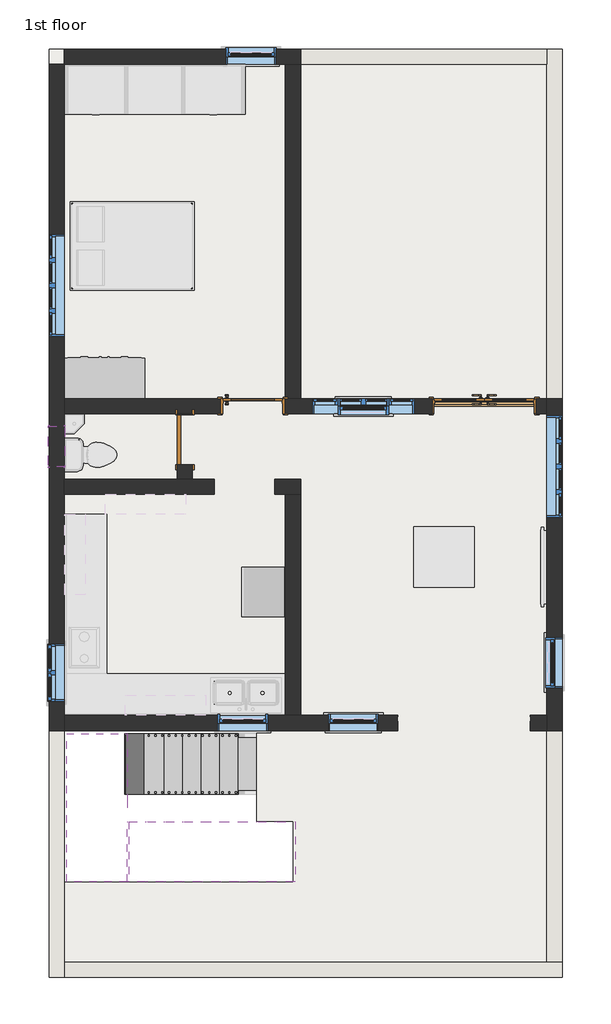
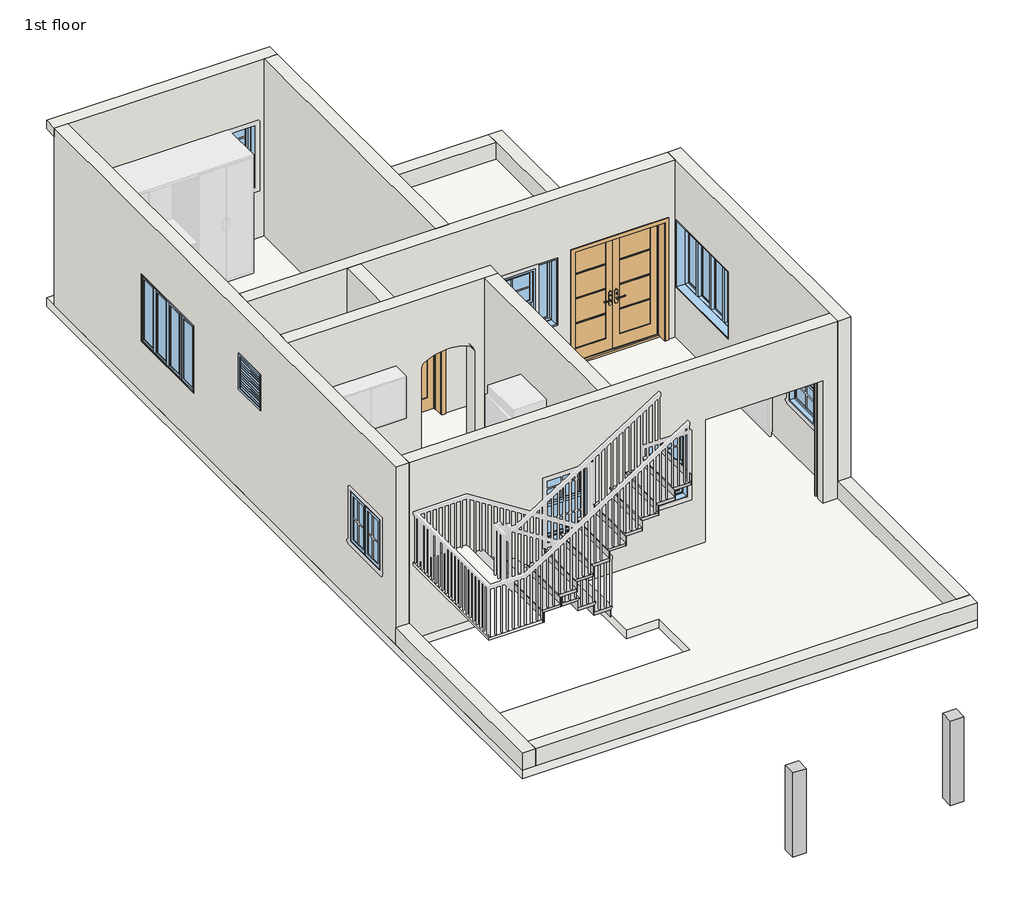
# One storey, part 1 of 3: 14 walls, 10 windows, 3 doors, 2 columns, 2 slabs, 2 stair flights.
"""IFC4 building model written with IfcOpenShell, lengths in millimetres."""

from ifc_helpers import new_model, si_unit, point, frame, origin, place, context, project, spatial, polyline, ellipse_curve, trimmed, outline, extrude, faceted_brep, transform, mapped, element, save
from ifc_brep_helpers import plane_surface, extruded_surface, advanced_brep
from components import concrete_square_column_fdf53bfc, door_7bc300fe, door_3b97b8e7, door_bb98abfd, non_monolithic_landing_a0269062, stair_flight_80511569, stair_flight_9ab9eb73, window_339605e1, window_cf6260c5, window_d400040f, window_913990a0, window_f2d8fef0

model = new_model("IFC4")

# Units and contexts
model_context = context("Model", 3, world=origin())
ifc_project = project(units=[si_unit("LENGTHUNIT", "METRE", prefix="MILLI")], contexts=[model_context])

# Site, building, storey
site = spatial("IfcSite", under=ifc_project)
building = spatial("IfcBuilding", under=site)
storey = spatial("IfcBuildingStorey", under=building, Name="1st floor", Elevation=3810.0)

# Columns
placement = place(None, origin())
concrete_square_column_shape = concrete_square_column_fdf53bfc(model_context)
element("IfcColumn", 1, ObjectType="Concrete-Square-Column", at=placement, inside=storey, context=model_context, shape_type="MappedRepresentation", body=[
    mapped(concrete_square_column_shape, transform((35811.8316163, 5713.6980552, 0.0), x_axis=(1.0, 0.0, 0.0), y_axis=(0.0, 1.0, 0.0), z_axis=(0.0, 0.0, 1.0))),
])
element("IfcColumn", 2, ObjectType="Concrete-Square-Column", at=placement, inside=storey, context=model_context, shape_type="MappedRepresentation", body=[
    mapped(concrete_square_column_shape, transform((33125.7468179, 5719.9369036, 0.0), x_axis=(1.0, 0.0, 0.0), y_axis=(0.0, 1.0, 0.0), z_axis=(0.0, 0.0, 1.0))),
])

# Doors
door_shape = door_7bc300fe(model_context)
element("IfcDoor", 3, ObjectType="Door-Exterior-Double-Full Glass-Wood_Clad : 60\" x 84\"", at=placement, inside=storey, context=model_context, shape_type="MappedRepresentation", body=[
    mapped(door_shape, transform((34973.6316163, 14251.2730552, 3810.0), x_axis=(-1.0, 0.0, 0.0), y_axis=(0.0, -1.0, 0.0), z_axis=(0.0, 0.0, 1.0))),
])
door_2_shape = door_3b97b8e7(model_context)
element("IfcDoor", 4, ObjectType="Door-Interior-Single-1_Panel-Wood : 36\" x 84\"", at=placement, inside=storey, context=model_context, shape_type="MappedRepresentation", body=[
    mapped(door_2_shape, transform((31468.4316163, 14251.2730552, 3810.0), x_axis=(1.0, 0.0, 0.0), y_axis=(0.0, 1.0, 0.0), z_axis=(0.0, 0.0, 1.0))),
])
door_3_shape = door_bb98abfd(model_context)
element("IfcDoor", 5, ObjectType="Single-Flush : 30\" x 84\"", at=placement, inside=storey, context=model_context, shape_type="MappedRepresentation", body=[
    mapped(door_3_shape, transform((30439.7316163, 13740.0980552, 3810.0), x_axis=(0.0, 1.0, 0.0), y_axis=(-1.0, 0.0, 0.0), z_axis=(0.0, 0.0, 1.0))),
])

# Slabs
element("IfcSlab", 6, ObjectType="Generic - 12\" 2", at=placement, inside=storey, context=model_context, shape_type="SweptSolid", body=[
    extrude(outline(polyline([(36154.7316163, 19658.2980552), (36154.7316163, 5593.0480552), (28382.3316163, 5593.0480552), (28382.3316163, 19658.2980552), (36154.7316163, 19658.2980552)]), holes=[polyline([(31519.2316163, 7955.2480552), (31519.2316163, 9333.1980552), (28610.9316163, 9333.1980552), (28610.9316163, 7040.8480552), (32078.0316163, 7040.8480552), (32078.0316163, 7955.2480552), (31519.2316163, 7955.2480552)])]), frame((0.0, 0.0, 3657.6), z_axis=(0.0, 0.0, 1.0), x_axis=(1.0, 0.0, 0.0)), (0.0, 0.0, 1.0), 152.4),
])
non_monolithic_landing_shape = non_monolithic_landing_a0269062(model_context)
element("IfcSlab", 7, ObjectType="Non-Monolithic Landing", at=placement, inside=storey, context=model_context, shape_type="MappedRepresentation", body=[
    mapped(non_monolithic_landing_shape, transform((0.0, 0.0, 0.0), x_axis=(1.0, 0.0, 0.0), y_axis=(0.0, 1.0, 0.0), z_axis=(0.0, 0.0, 1.0))),
])

# Stair flights
stair_flight_shape = stair_flight_80511569(model_context)
element("IfcStairFlight", 8, ObjectType="2\" Tread 1\" Nosing 1/4\" Riser", at=placement, inside=storey, context=model_context, shape_type="MappedRepresentation", body=[
    mapped(stair_flight_shape, transform((0.0, 0.0, 0.0), x_axis=(1.0, 0.0, 0.0), y_axis=(0.0, 1.0, 0.0), z_axis=(0.0, 0.0, 1.0))),
])
stair_flight_2_shape = stair_flight_9ab9eb73(model_context)
element("IfcStairFlight", 9, ObjectType="2\" Tread 1\" Nosing 1/4\" Riser", at=placement, inside=storey, context=model_context, shape_type="MappedRepresentation", body=[
    mapped(stair_flight_2_shape, transform((0.0, 0.0, 0.0), x_axis=(1.0, 0.0, 0.0), y_axis=(0.0, 1.0, 0.0), z_axis=(0.0, 0.0, 1.0))),
])

# Walls
element("IfcWall", 10, ObjectType="Generic - 9\"", at=placement, inside=storey, context=model_context, shape_type="Brep", body=[
    faceted_brep([(28610.9316163, 19429.6980552, 3810.0), (31963.7316163, 19429.6980552, 3810.0), (32192.3316163, 19429.6980552, 3810.0), (32192.3316163, 19429.6980552, 4114.8), (32192.3316163, 19429.6980552, 7010.4), (31963.7316163, 19429.6980552, 7010.4), (28610.9316163, 19429.6980552, 7010.4), (28382.3316163, 19429.6980552, 7010.4), (28382.3316163, 19429.6980552, 6858.0), (28610.9316163, 19429.6980552, 6858.0), (31062.0316163, 19429.6980552, 5892.8), (31824.0316163, 19429.6980552, 5892.8), (31824.0316163, 19429.6980552, 4724.4), (31062.0316163, 19429.6980552, 4724.4), (28610.9316163, 19658.2980552, 3810.0), (28610.9316163, 19658.2980552, 6858.0), (28382.3316163, 19658.2980552, 6858.0), (28382.3316163, 19658.2980552, 7010.4), (32192.3316163, 19658.2980552, 7010.4), (32192.3316163, 19658.2980552, 4114.8), (32192.3316163, 19658.2980552, 3810.0), (31062.0316163, 19658.2980552, 5892.8), (31062.0316163, 19658.2980552, 4724.4), (31824.0316163, 19658.2980552, 4724.4), (31824.0316163, 19658.2980552, 5892.8)], [[[0, 1, 2, 3, 4, 5, 6, 7, 8, 9], [10, 11, 12, 13]], [[14, 15, 16, 17, 18, 19, 20], [21, 22, 23, 24]], [[2, 1, 0, 14, 20]], [[7, 6, 5, 4, 18, 17]], [[22, 21, 10, 13]], [[23, 22, 13, 12]], [[24, 23, 12, 11]], [[21, 24, 11, 10]], [[2, 20, 19, 18, 4, 3]], [[8, 16, 15, 9]], [[0, 9, 15, 14]], [[8, 7, 17, 16]]]),
])
element("IfcWall", 11, ObjectType="Generic - 9\"", at=placement, inside=storey, context=model_context, shape_type="Brep", body=[
    faceted_brep([(35926.1316163, 14133.7980552, 7010.4), (30554.0316163, 14133.7980552, 7010.4), (30325.4316163, 14133.7980552, 7010.4), (28610.9316163, 14133.7980552, 7010.4), (28610.9316163, 14133.7980552, 3810.0), (30325.4316163, 14133.7980552, 3810.0), (30554.0316163, 14133.7980552, 3810.0), (30985.8316163, 14133.7980552, 3810.0), (30985.8316163, 14133.7980552, 5969.0), (31951.0316163, 14133.7980552, 5969.0), (31951.0316163, 14133.7980552, 3810.0), (34186.2316163, 14133.7980552, 3810.0), (34186.2316163, 14133.7980552, 5969.0), (35761.0316163, 14133.7980552, 5969.0), (35761.0316163, 14133.7980552, 3810.0), (35926.1316163, 14133.7980552, 3810.0), (33919.5316163, 14133.7980552, 4724.4), (32370.1316163, 14133.7980552, 4724.4), (32370.1316163, 14133.7980552, 5943.6), (33919.5316163, 14133.7980552, 5943.6), (28610.9316163, 14362.3980552, 7010.4), (31963.7316163, 14362.3980552, 7010.4), (32192.3316163, 14362.3980552, 7010.4), (35926.1316163, 14362.3980552, 7010.4), (35926.1316163, 14362.3980552, 6858.0), (35926.1316163, 14362.3980552, 3810.0), (35761.0316163, 14362.3980552, 3810.0), (35761.0316163, 14362.3980552, 5969.0), (34186.2316163, 14362.3980552, 5969.0), (34186.2316163, 14362.3980552, 3810.0), (32192.3316163, 14362.3980552, 3810.0), (31963.7316163, 14362.3980552, 3810.0), (31951.0316163, 14362.3980552, 3810.0), (31951.0316163, 14362.3980552, 5969.0), (30985.8316163, 14362.3980552, 5969.0), (30985.8316163, 14362.3980552, 3810.0), (28610.9316163, 14362.3980552, 3810.0), (32370.1316163, 14362.3980552, 4724.4), (33919.5316163, 14362.3980552, 4724.4), (33919.5316163, 14362.3980552, 5943.6), (32370.1316163, 14362.3980552, 5943.6)], [[[0, 1, 2, 3, 4, 5, 6, 7, 8, 9, 10, 11, 12, 13, 14, 15], [16, 17, 18, 19]], [[20, 21, 22, 23, 24, 25, 26, 27, 28, 29, 30, 31, 32, 33, 34, 35, 36], [37, 38, 39, 40]], [[4, 36, 35, 7, 6, 5]], [[15, 14, 26, 25]], [[29, 11, 10, 32, 31, 30]], [[3, 2, 1, 0, 23, 22, 21, 20]], [[37, 17, 16, 38]], [[28, 12, 11, 29]], [[12, 28, 27, 13]], [[13, 27, 26, 14]], [[9, 33, 32, 10]], [[33, 9, 8, 34]], [[34, 8, 7, 35]], [[19, 39, 38, 16]], [[17, 37, 40, 18]], [[39, 19, 18, 40]], [[15, 25, 24, 23, 0]], [[3, 20, 36, 4]]]),
])
element("IfcWall", 12, ObjectType="Generic - 9\"", at=placement, inside=storey, context=model_context, shape_type="AdvancedBrep", body=[
    advanced_brep(
    [(28610.9316163, 12914.5980552, 3810.0), (30884.2316163, 12914.5980552, 3810.0), (30884.2316163, 12914.5980552, 5740.4), (31798.6316163, 12914.5980552, 5740.4), (31798.6316163, 12914.5980552, 3810.0), (31963.7316163, 12914.5980552, 3810.0), (32192.3316163, 12914.5980552, 3810.0), (32192.3316163, 12914.5980552, 6858.0), (32192.3316163, 12914.5980552, 7010.4), (31963.7316163, 12914.5980552, 7010.4), (28610.9316163, 12914.5980552, 7010.4), (30884.2316163, 13143.1980552, 5740.4), (30884.2316163, 13143.1980552, 3810.0), (30554.0316163, 13143.1980552, 3810.0), (30325.4316163, 13143.1980552, 3810.0), (28610.9316163, 13143.1980552, 3810.0), (28610.9316163, 13143.1980552, 7010.4), (30325.4316163, 13143.1980552, 7010.4), (30554.0316163, 13143.1980552, 7010.4), (32192.3316163, 13143.1980552, 7010.4), (32192.3316163, 13143.1980552, 3810.0), (31963.7316163, 13143.1980552, 3810.0), (31798.6316163, 13143.1980552, 3810.0), (31798.6316163, 13143.1980552, 5740.4)],
    [
        (0, 1),
        (1, 2),
        (2, 3, ellipse_curve(frame((31341.4316163, 12914.5980552, 5740.4), z_axis=(0.0, 1.0, 0.0), x_axis=(-1.0, 0.0, 0.0)), 457.2, 203.2)),
        (3, 4),
        (4, 5),
        (5, 6),
        (6, 7),
        (7, 8),
        (8, 9),
        (9, 10),
        (10, 0),
        (11, 12),
        (12, 13),
        (13, 14),
        (14, 15),
        (15, 16),
        (16, 17),
        (17, 18),
        (18, 19),
        (19, 20),
        (20, 21),
        (21, 22),
        (22, 23),
        (23, 11, ellipse_curve(frame((31341.4316163, 13143.1980552, 5740.4), z_axis=(0.0, -1.0, 0.0), x_axis=(-1.0, 0.0, 0.0)), 457.2, 203.2)),
        (12, 1),
        (0, 15),
        (20, 6),
        (4, 22),
        (8, 19),
        (16, 10),
        (2, 11),
        (23, 3),
    ],
    [
        plane_surface(frame((28648.9011308, 12914.5980552, 3810.0), z_axis=(0.0, -1.0, 0.0), x_axis=(1.0, 0.0, 0.0))),
        plane_surface(frame((28648.9011308, 13143.1980552, 3810.0), z_axis=(0.0, 1.0, 0.0), x_axis=(-1.0, 0.0, 0.0))),
        plane_surface(frame((28496.6316163, 12914.5980552, 3810.0), z_axis=(0.0, 0.0, -1.0), x_axis=(0.0, 1.0, 0.0))),
        plane_surface(frame((32078.0316163, 12914.5980552, 7010.4), z_axis=(0.0, 0.0, 1.0), x_axis=(0.0, 1.0, 0.0))),
        plane_surface(frame((28610.9316163, 5713.6980552, 3810.0), z_axis=(-1.0, 0.0, 0.0), x_axis=(0.0, 1.0, 0.0))),
        extruded_surface(trimmed(ellipse_curve(frame((31341.4316163, 13371.7980552, 5740.4), z_axis=(0.0, 1.0, 0.0), x_axis=(-1.0, 0.0, 0.0)), 457.2, 203.2), [point((30884.2316163, 13371.7980552, 5740.4))], [point((31798.6316163, 13371.7980552, 5740.4))], True, "CARTESIAN"), (0.0, -228.60000000000036, 0.0), 228.60000000000036),
        plane_surface(frame((31798.6316163, 12914.5980552, 5740.4), z_axis=(-1.0, 0.0, 0.0), x_axis=(0.0, 1.0, 0.0))),
        plane_surface(frame((30884.2316163, 12914.5980552, 3810.0), z_axis=(1.0, 0.0, 0.0), x_axis=(0.0, 1.0, 0.0))),
        plane_surface(frame((32192.3316163, 9561.7980552, 3810.0), z_axis=(1.0, 0.0, 0.0), x_axis=(0.0, 1.0, 0.0))),
    ],
    [
        (0, [[1, 2, 3, 4, 5, 6, 7, 8, 9, 10, 11]]),
        (1, [[12, 13, 14, 15, 16, 17, 18, 19, 20, 21, 22, 23, 24]]),
        (2, [[-15, -14, -13, 25, -1, 26]]),
        (2, [[-22, -21, 27, -6, -5, 28]]),
        (3, [[-10, -9, 29, -19, -18, -17, 30]]),
        (4, [[-11, -30, -16, -26]]),
        (5, [[-3, 31, -24, 32]]),
        (6, [[-4, -32, -23, -28]]),
        (7, [[-2, -25, -12, -31]]),
        (8, [[-27, -20, -29, -8, -7]]),
    ],
),
])
element("IfcWall", 13, ObjectType="Generic - 9\"", at=placement, inside=storey, context=model_context, shape_type="Brep", body=[
    faceted_brep([(35926.1316163, 9333.1980552, 7010.4), (28610.9316163, 9333.1980552, 7010.4), (28610.9316163, 9333.1980552, 3810.0), (33668.8316163, 9333.1980552, 3810.0), (33668.8316163, 9333.1980552, 6019.0), (35668.8316163, 9333.1980552, 6019.0), (35668.8316163, 9333.1980552, 3810.0), (35926.1316163, 9333.1980552, 3810.0), (32611.4316163, 9333.1980552, 5892.8), (33373.4316163, 9333.1980552, 5892.8), (33373.4316163, 9333.1980552, 4724.4), (32611.4316163, 9333.1980552, 4724.4), (30935.0316163, 9333.1980552, 5892.8), (31697.0316163, 9333.1980552, 5892.8), (31697.0316163, 9333.1980552, 4724.4), (30935.0316163, 9333.1980552, 4724.4), (28610.9316163, 9561.7980552, 7010.4), (31963.7316163, 9561.7980552, 7010.4), (32192.3316163, 9561.7980552, 7010.4), (35926.1316163, 9561.7980552, 7010.4), (35926.1316163, 9561.7980552, 3810.0), (35668.8316163, 9561.7980552, 3810.0), (35668.8316163, 9561.7980552, 6019.0), (33668.8316163, 9561.7980552, 6019.0), (33668.8316163, 9561.7980552, 3810.0), (32192.3316163, 9561.7980552, 3810.0), (31963.7316163, 9561.7980552, 3810.0), (28610.9316163, 9561.7980552, 3810.0), (32611.4316163, 9561.7980552, 5892.8), (32611.4316163, 9561.7980552, 4724.4), (33373.4316163, 9561.7980552, 4724.4), (33373.4316163, 9561.7980552, 5892.8), (30935.0316163, 9561.7980552, 5892.8), (30935.0316163, 9561.7980552, 4724.4), (31697.0316163, 9561.7980552, 4724.4), (31697.0316163, 9561.7980552, 5892.8), (33668.8316163, 9541.7980552, 3810.0), (33653.8316163, 9541.7980552, 3810.0), (33653.8316163, 9471.7980552, 3810.0), (33668.8316163, 9471.7980552, 3810.0), (35668.8316163, 9471.7980552, 3810.0), (35683.8316163, 9471.7980552, 3810.0), (35683.8316163, 9541.7980552, 3810.0), (35668.8316163, 9541.7980552, 3810.0), (35668.8316163, 9541.7980552, 6019.0), (33668.8316163, 9541.7980552, 6019.0), (33668.8316163, 9471.7980552, 6019.0), (35668.8316163, 9471.7980552, 6019.0), (33653.8316163, 9471.7980552, 6034.0), (35683.8316163, 9471.7980552, 6034.0), (33653.8316163, 9541.7980552, 6034.0), (35683.8316163, 9541.7980552, 6034.0)], [[[0, 1, 2, 3, 4, 5, 6, 7], [8, 9, 10, 11], [12, 13, 14, 15]], [[16, 17, 18, 19, 20, 21, 22, 23, 24, 25, 26, 27], [28, 29, 30, 31], [32, 33, 34, 35]], [[2, 27, 26, 25, 24, 36, 37, 38, 39, 3]], [[20, 7, 6, 40, 41, 42, 43, 21]], [[1, 0, 19, 18, 17, 16]], [[44, 45, 23, 22]], [[46, 47, 5, 4]], [[47, 40, 6, 5]], [[39, 46, 4, 3]], [[47, 46, 39, 38, 48, 49, 41, 40]], [[48, 38, 37, 50]], [[45, 44, 43, 42, 51, 50, 37, 36]], [[45, 36, 24, 23]], [[43, 44, 22, 21]], [[41, 49, 51, 42]], [[49, 48, 50, 51]], [[29, 28, 8, 11]], [[30, 29, 11, 10]], [[31, 30, 10, 9]], [[28, 31, 9, 8]], [[33, 32, 12, 15]], [[34, 33, 15, 14]], [[35, 34, 14, 13]], [[32, 35, 13, 12]], [[27, 2, 1, 16]], [[7, 20, 19, 0]]]),
])
element("IfcWall", 14, ObjectType="Generic - 9\"", at=placement, inside=storey, context=model_context, shape_type="SweptSolid", body=[
    extrude(outline(polyline([(32192.3316163, 12914.5980552), (32192.3316163, 9561.7980552), (31963.7316163, 9561.7980552), (31963.7316163, 12914.5980552), (32192.3316163, 12914.5980552)])), frame((0.0, 0.0, 3810.0), z_axis=(0.0, 0.0, 1.0), x_axis=(1.0, 0.0, 0.0)), (0.0, 0.0, 1.0), 3200.4),
])
element("IfcWall", 15, ObjectType="Generic - 9\"", at=placement, inside=storey, context=model_context, shape_type="SweptSolid", body=[
    extrude(outline(polyline([(14133.7980552, 3810.0), (14121.0980552, 3810.0), (14121.0980552, 5943.6), (13359.0980552, 5943.6), (13359.0980552, 3810.0), (13143.1980552, 3810.0), (13143.1980552, 7010.4), (14133.7980552, 7010.4), (14133.7980552, 3810.0)])), frame((30325.4316163, 0.0, 0.0), z_axis=(1.0, 0.0, 0.0), x_axis=(0.0, 1.0, 0.0)), (0.0, 0.0, 1.0), 228.6),
])
element("IfcWall", 16, ObjectType="Generic - 9\"", at=placement, inside=storey, context=model_context, shape_type="Brep", body=[
    faceted_brep([(28610.9316163, 9333.1980552, 7010.4), (28610.9316163, 9333.1980552, 6858.0), (28610.9316163, 9333.1980552, 4114.8), (28610.9316163, 9333.1980552, 3810.0), (28610.9316163, 9561.7980552, 3810.0), (28610.9316163, 12914.5980552, 3810.0), (28610.9316163, 13143.1980552, 3810.0), (28610.9316163, 14133.7980552, 3810.0), (28610.9316163, 14362.3980552, 3810.0), (28610.9316163, 19429.6980552, 3810.0), (28610.9316163, 19429.6980552, 7010.4), (28610.9316163, 14362.3980552, 7010.4), (28610.9316163, 14133.7980552, 7010.4), (28610.9316163, 13143.1980552, 7010.4), (28610.9316163, 12914.5980552, 7010.4), (28610.9316163, 9561.7980552, 7010.4), (28610.9316163, 13333.6980552, 6248.4), (28610.9316163, 13943.2980552, 6248.4), (28610.9316163, 13943.2980552, 5638.8), (28610.9316163, 13333.6980552, 5638.8), (28610.9316163, 16851.5980552, 5943.6), (28610.9316163, 16851.5980552, 4724.4), (28610.9316163, 15302.1980552, 4724.4), (28610.9316163, 15302.1980552, 5943.6), (28610.9316163, 10641.2980552, 5803.9), (28610.9316163, 10641.2980552, 4889.5), (28610.9316163, 9777.6980552, 4889.5), (28610.9316163, 9777.6980552, 5803.9), (28382.3316163, 9333.1980552, 3810.0), (28382.3316163, 9333.1980552, 4114.8), (28382.3316163, 9333.1980552, 7010.4), (28382.3316163, 19429.6980552, 7010.4), (28382.3316163, 19429.6980552, 6858.0), (28382.3316163, 19429.6980552, 3810.0), (28382.3316163, 9561.7980552, 3810.0), (28382.3316163, 13333.6980552, 6248.4), (28382.3316163, 13333.6980552, 5638.8), (28382.3316163, 13943.2980552, 5638.8), (28382.3316163, 13943.2980552, 6248.4), (28382.3316163, 16851.5980552, 5943.6), (28382.3316163, 15302.1980552, 5943.6), (28382.3316163, 15302.1980552, 4724.4), (28382.3316163, 16851.5980552, 4724.4), (28382.3316163, 10641.2980552, 5803.9), (28382.3316163, 9777.6980552, 5803.9), (28382.3316163, 9777.6980552, 4889.5), (28382.3316163, 10641.2980552, 4889.5)], [[[0, 1, 2, 3, 4, 5, 6, 7, 8, 9, 10, 11, 12, 13, 14, 15], [16, 17, 18, 19], [20, 21, 22, 23], [24, 25, 26, 27]], [[28, 29, 30, 31, 32, 33, 34], [35, 36, 37, 38], [39, 40, 41, 42], [43, 44, 45, 46]], [[9, 8, 7, 6, 5, 4, 3, 28, 34, 33]], [[0, 15, 14, 13, 12, 11, 10, 31, 30]], [[36, 35, 16, 19]], [[37, 36, 19, 18]], [[38, 37, 18, 17]], [[35, 38, 17, 16]], [[21, 20, 39, 42]], [[22, 21, 42, 41]], [[23, 22, 41, 40]], [[20, 23, 40, 39]], [[25, 24, 43, 46]], [[26, 25, 46, 45]], [[27, 26, 45, 44]], [[24, 27, 44, 43]], [[0, 30, 29, 28, 3, 2, 1]], [[9, 33, 32, 31, 10]]]),
])
element("IfcWall", 17, ObjectType="Generic - 9\"", at=placement, inside=storey, context=model_context, shape_type="SweptSolid", body=[
    extrude(outline(polyline([(32192.3316163, 19429.6980552), (32192.3316163, 14362.3980552), (31963.7316163, 14362.3980552), (31963.7316163, 19429.6980552), (32192.3316163, 19429.6980552)])), frame((0.0, 0.0, 3810.0), z_axis=(0.0, 0.0, 1.0), x_axis=(1.0, 0.0, 0.0)), (0.0, 0.0, 1.0), 3200.4),
])
element("IfcWall", 18, ObjectType="Generic - 9\"", at=placement, inside=storey, context=model_context, shape_type="Brep", body=[
    faceted_brep([(35926.1316163, 14362.3980552, 7010.4), (35926.1316163, 14362.3980552, 6858.0), (35926.1316163, 14362.3980552, 4114.8), (35926.1316163, 14362.3980552, 3810.0), (35926.1316163, 14133.7980552, 3810.0), (35926.1316163, 9561.7980552, 3810.0), (35926.1316163, 9333.1980552, 3810.0), (35926.1316163, 9333.1980552, 4114.8), (35926.1316163, 9333.1980552, 6858.0), (35926.1316163, 9333.1980552, 7010.4), (35926.1316163, 9561.7980552, 7010.4), (35926.1316163, 14133.7980552, 7010.4), (35926.1316163, 9980.8980552, 5892.8), (35926.1316163, 9980.8980552, 4724.4), (35926.1316163, 10742.8980552, 4724.4), (35926.1316163, 10742.8980552, 5892.8), (35926.1316163, 12558.9980552, 5943.6), (35926.1316163, 12558.9980552, 4724.4), (35926.1316163, 14108.3980552, 4724.4), (35926.1316163, 14108.3980552, 5943.6), (36154.7316163, 14362.3980552, 3810.0), (36154.7316163, 14362.3980552, 4114.8), (36154.7316163, 14362.3980552, 7010.4), (36154.7316163, 9333.1980552, 7010.4), (36154.7316163, 9333.1980552, 4114.8), (36154.7316163, 9333.1980552, 3810.0), (36154.7316163, 9561.7980552, 3810.0), (36154.7316163, 9980.8980552, 5892.8), (36154.7316163, 10742.8980552, 5892.8), (36154.7316163, 10742.8980552, 4724.4), (36154.7316163, 9980.8980552, 4724.4), (36154.7316163, 12558.9980552, 5943.6), (36154.7316163, 14108.3980552, 5943.6), (36154.7316163, 14108.3980552, 4724.4), (36154.7316163, 12558.9980552, 4724.4)], [[[0, 1, 2, 3, 4, 5, 6, 7, 8, 9, 10, 11], [12, 13, 14, 15], [16, 17, 18, 19]], [[20, 21, 22, 23, 24, 25, 26], [27, 28, 29, 30], [31, 32, 33, 34]], [[6, 5, 4, 3, 20, 26, 25]], [[0, 11, 10, 9, 23, 22]], [[12, 15, 28, 27]], [[15, 14, 29, 28]], [[14, 13, 30, 29]], [[13, 12, 27, 30]], [[16, 19, 32, 31]], [[19, 18, 33, 32]], [[18, 17, 34, 33]], [[17, 16, 31, 34]], [[6, 25, 24, 23, 9, 8, 7]], [[0, 22, 21, 20, 3, 2, 1]]]),
])
element("IfcWall", 19, ObjectType="Generic - 9\"", at=placement, inside=storey, context=model_context, shape_type="Brep", body=[
    faceted_brep([(28382.3316163, 9333.1980552, 3810.0), (28382.3316163, 5593.0480552, 3810.0), (28382.3316163, 5593.0480552, 4114.8), (28382.3316163, 9333.1980552, 4114.8), (28610.9316163, 9333.1980552, 3810.0), (28610.9316163, 9333.1980552, 4114.8), (28610.9316163, 5821.6480552, 4114.8), (28610.9316163, 5593.0480552, 4114.8), (28610.9316163, 5593.0480552, 3810.0), (28610.9316163, 5821.6480552, 3810.0)], [[[0, 1, 2, 3]], [[4, 5, 6, 7, 8, 9]], [[1, 0, 4, 9, 8]], [[3, 2, 7, 6, 5]], [[2, 1, 8, 7]], [[0, 3, 5, 4]]]),
])
element("IfcWall", 20, ObjectType="Generic - 9\"", at=placement, inside=storey, context=model_context, shape_type="Brep", body=[
    faceted_brep([(28610.9316163, 5593.0480552, 3810.0), (36154.7316163, 5593.0480552, 3810.0), (36154.7316163, 5593.0480552, 4114.8), (28610.9316163, 5593.0480552, 4114.8), (28610.9316163, 5821.6480552, 3810.0), (28610.9316163, 5821.6480552, 4114.8), (35926.1316163, 5821.6480552, 4114.8), (36154.7316163, 5821.6480552, 4114.8), (36154.7316163, 5821.6480552, 3810.0), (35926.1316163, 5821.6480552, 3810.0)], [[[0, 1, 2, 3]], [[4, 5, 6, 7, 8, 9]], [[1, 0, 4, 9, 8]], [[3, 2, 7, 6, 5]], [[0, 3, 5, 4]], [[2, 1, 8, 7]]]),
])
element("IfcWall", 21, ObjectType="Generic - 9\"", at=placement, inside=storey, context=model_context, shape_type="SweptSolid", body=[
    extrude(outline(polyline([(36154.7316163, 9333.1980552), (36154.7316163, 5821.6480552), (35926.1316163, 5821.6480552), (35926.1316163, 9333.1980552), (36154.7316163, 9333.1980552)])), frame((0.0, 0.0, 3810.0), z_axis=(0.0, 0.0, 1.0), x_axis=(1.0, 0.0, 0.0)), (0.0, 0.0, 1.0), 304.8),
])
element("IfcWall", 22, ObjectType="Generic - 9\"", at=placement, inside=storey, context=model_context, shape_type="Brep", body=[
    faceted_brep([(36154.7316163, 14362.3980552, 3810.0), (36154.7316163, 19429.6980552, 3810.0), (36154.7316163, 19658.2980552, 3810.0), (36154.7316163, 19658.2980552, 4114.8), (36154.7316163, 14362.3980552, 4114.8), (35926.1316163, 14362.3980552, 3810.0), (35926.1316163, 14362.3980552, 4114.8), (35926.1316163, 19429.6980552, 4114.8), (35926.1316163, 19658.2980552, 4114.8), (35926.1316163, 19658.2980552, 3810.0), (35926.1316163, 19429.6980552, 3810.0)], [[[0, 1, 2, 3, 4]], [[5, 6, 7, 8, 9, 10]], [[2, 1, 0, 5, 10, 9]], [[4, 3, 8, 7, 6]], [[3, 2, 9, 8]], [[0, 4, 6, 5]]]),
])
element("IfcWall", 23, ObjectType="Generic - 9\"", at=placement, inside=storey, context=model_context, shape_type="SweptSolid", body=[
    extrude(outline(polyline([(32192.3316163, 19658.2980552), (35926.1316163, 19658.2980552), (35926.1316163, 19429.6980552), (32192.3316163, 19429.6980552), (32192.3316163, 19658.2980552)])), frame((0.0, 0.0, 3810.0), z_axis=(0.0, 0.0, 1.0), x_axis=(1.0, 0.0, 0.0)), (0.0, 0.0, 1.0), 304.8),
])

# Windows
window_shape = window_339605e1(model_context)
element("IfcWindow", 24, ObjectType="Window-Casement-Double : 34\" x 36\"", at=placement, inside=storey, context=model_context, shape_type="MappedRepresentation", body=[
    mapped(window_shape, transform((28496.6316163, 10209.4980552, 3975.1), x_axis=(0.0, 1.0, 0.0), y_axis=(-1.0, 0.0, 0.0), z_axis=(0.0, 0.0, 1.0))),
])
window_2_shape = window_cf6260c5(model_context)
element("IfcWindow", 25, ObjectType="Window-Casement-Multi-Sash-Horizontal : 61\" x 48\"", at=placement, inside=storey, context=model_context, shape_type="MappedRepresentation", body=[
    mapped(window_2_shape, transform((28496.6316163, 16076.8980552, 3810.0), x_axis=(0.0, 1.0, 0.0), y_axis=(-1.0, 0.0, 0.0), z_axis=(0.0, 0.0, 1.0))),
])
element("IfcWindow", 26, ObjectType="Window-Casement-Multi-Sash-Horizontal : 61\" x 48\"", at=placement, inside=storey, context=model_context, shape_type="MappedRepresentation", body=[
    mapped(window_2_shape, transform((33144.8316163, 14248.0980552, 3810.0), x_axis=(1.0, 0.0, 0.0), y_axis=(0.0, 1.0, 0.0), z_axis=(0.0, 0.0, 1.0))),
])
element("IfcWindow", 27, ObjectType="Window-Casement-Multi-Sash-Horizontal : 61\" x 48\"", at=placement, inside=storey, context=model_context, shape_type="MappedRepresentation", body=[
    mapped(window_2_shape, transform((36040.4316163, 13333.6980552, 3810.0), x_axis=(0.0, -1.0, 0.0), y_axis=(1.0, 0.0, 0.0), z_axis=(0.0, 0.0, 1.0))),
])
window_3_shape = window_d400040f(model_context)
element("IfcWindow", 28, ObjectType="Window-Double-Hung : 30\" x 46\"", at=placement, inside=storey, context=model_context, shape_type="MappedRepresentation", body=[
    mapped(window_3_shape, transform((32992.4316163, 9447.4980552, 3810.0), x_axis=(1.0, 0.0, 0.0), y_axis=(0.0, 1.0, 0.0), z_axis=(0.0, 0.0, 1.0))),
])
element("IfcWindow", 29, ObjectType="Window-Double-Hung : 30\" x 46\"", at=placement, inside=storey, context=model_context, shape_type="MappedRepresentation", body=[
    mapped(window_3_shape, transform((31316.0316163, 9447.4980552, 3810.0), x_axis=(1.0, 0.0, 0.0), y_axis=(0.0, 1.0, 0.0), z_axis=(0.0, 0.0, 1.0))),
])
element("IfcWindow", 30, ObjectType="Window-Double-Hung : 30\" x 46\"", at=placement, inside=storey, context=model_context, shape_type="MappedRepresentation", body=[
    mapped(window_3_shape, transform((36040.4316163, 10361.8980552, 3810.0), x_axis=(0.0, 1.0, 0.0), y_axis=(-1.0, 0.0, 0.0), z_axis=(0.0, 0.0, 1.0))),
])
element("IfcWindow", 31, ObjectType="Window-Double-Hung : 30\" x 46\"", at=placement, inside=storey, context=model_context, shape_type="MappedRepresentation", body=[
    mapped(window_3_shape, transform((31443.0316163, 19543.9980552, 3810.0), x_axis=(1.0, 0.0, 0.0), y_axis=(0.0, 1.0, 0.0), z_axis=(0.0, 0.0, 1.0))),
])
window_4_shape = window_913990a0(model_context)
element("IfcWindow", 32, ObjectType="Window-Double-Hung : 30\" x 46\"", at=placement, inside=storey, context=model_context, shape_type="MappedRepresentation", body=[
    mapped(window_4_shape, transform((33144.8316163, 14248.0980552, 3810.0), x_axis=(1.0, 0.0, 0.0), y_axis=(0.0, 1.0, 0.0), z_axis=(0.0, 0.0, 1.0))),
])
window_5_shape = window_f2d8fef0(model_context)
element("IfcWindow", 33, ObjectType="Window-Louvers : 24\" x 24\"", at=placement, inside=storey, context=model_context, shape_type="MappedRepresentation", body=[
    mapped(window_5_shape, transform((28490.2816163, 13638.4980552, 4724.4), x_axis=(0.0, 1.0, 0.0), y_axis=(-1.0, 0.0, 0.0), z_axis=(0.0, 0.0, 1.0))),
])

save(model, "model.ifc")

# Revit data of these elements
# Type "Concrete-Square-Column"
#   Assembly Code = "B10"
#   b = 0' - 9"
#   Structural Material [instance default] = Concrete, Cast-in-Place gray
# Type "Door-Exterior-Double-Full Glass-Wood_Clad : 60\" x 84\""
#   Type Mark = "9"
#   Assembly Code = "B2030100"
#   Analytic Construction = "French door, wood frame with double glass"
#   Top Rail = 0' - 4 11/16"
#   Threshold Offset [instance default] = 0' - 0 1/2"
#   Thickness = 0' - 1 3/8"
#   Thermal Resistance (R) = 1.9158 (h·ft²·°F)/BTU
#   Swing Angle [instance default] = 90.00°
#   Stiles = 0' - 4 3/4"
#   Rough Width = 5' - 2"
#   Rough Height = 7' - 1"
#   Panel Width = 2' - 6"
#   Door Offset [instance default] = 0' - 0"
#   Height = 7' - 0"
#   Width = 5' - 0"
#   Heat Transfer Coefficient (U) = 0.5220 BTU/(h·ft²·°F)
#   Bottom Rail = 0' - 9 1/8"
#   Exterior Trim [instance default] = yes
#   Threshold [instance default] = yes
#   Show Grill [instance default] = yes
#   Function = 1
#   Trim Material = Cherry
#   Threshold Material = Cherry
#   Panel Material = Cherry
#   Glazing = Glass
#   Frame Material = Cherry
#   Door Handle Material = Aluminum
#   Visual Light Transmittance = 0
#   Solar Heat Gain Coefficient = 0
#   Wall Closure = (empty or 0)
#   Construction Type = (empty or 0)
# Type "Door-Interior-Single-1_Panel-Wood : 36\" x 84\""
#   Type Mark = "8"
#   Assembly Code = "C1020300"
#   Analytic Construction = "Wooden"
#   Top Rail = 0' - 4 11/16"
#   Thickness = 0' - 1 3/8"
#   Thermal Resistance (R) = 2.5876 (h·ft²·°F)/BTU
#   Swing Angle [instance default] = 90.00°
#   Stiles = 0' - 4 3/4"
#   Rough Width = 3' - 2"
#   Rough Height = 7' - 1"
#   Height = 7' - 0"
#   Width = 3' - 0"
#   Heat Transfer Coefficient (U) = 0.3865 BTU/(h·ft²·°F)
#   Bottom Rail = 0' - 9 1/8"
#   Trim Material = Cherry
#   Panel Material = Cherry
#   Frame Material = Cherry
#   Door Handle Material = Aluminum
#   Visual Light Transmittance = 0
#   Solar Heat Gain Coefficient = 0
#   Wall Closure = (empty or 0)
#   Function = (empty or 0)
# Type "Single-Flush : 30\" x 84\""
#   Type Mark = "4"
#   Construction Type Id = "MDOOR"
#   Assembly Code = "C1020"
#   Analytic Construction = "Metal"
#   Thickness = 0' - 2"
#   Heat Transfer Coefficient (U) = 0.651978 BTU/(h·ft²·°F)
#   Height = 7' - 0"
#   Trim Projection Ext = 0' - 1"
#   Trim Projection Int = 0' - 1"
#   Trim Width = 0' - 3"
#   Width = 2' - 6"
#   Define Thermal Properties by = 1
#   Define Thermal Properties by = 1
#   Door Material = Door - Panel
#   Frame Material = Door - Frame
#   Visual Light Transmittance = 0
#   Solar Heat Gain Coefficient = 0
#   Function = (empty or 0)
#   Wall Closure = (empty or 0)
# Type "Generic - 12\" 2"
#   Assembly Code = "B1010"
#   Function = 0
#   Layers, outside or top first: 0' - 6" no material (function 1)
# Type "Generic - 9\""
#   Assembly Code = "B2010"
#   Layers, outside or top first: 0' - 9" no material (function 1)
# Type "Window-Casement-Double : 34\" x 36\""
#   Type Mark = "14"
#   Fire Rating = "0.5h"
#   Assembly Code = "B2020100"
#   Analytic Construction = "Double glazing - domestic"
#   Frame Extension [instance default] = 0' - 0 1/4"
#   Window Inset [instance default] = 0' - 0"
#   Wall Thickness [instance default] = 0' - 6"
#   Interior Wall Closure [instance default] = 0' - 2 1/4"
#   Half Width = 1' - 5"
#   Visual Light Transmittance = 0.81
#   Thermal Resistance (R) = 1.8146 (h·ft²·°F)/BTU
#   Solar Heat Gain Coefficient = 0.76
#   Rough Width = 2' - 10 1/2"
#   Rough Height = 3' - 0 1/2"
#   Height = 3' - 0"
#   Heat Transfer Coefficient (U) = 0.5511 BTU/(h·ft²·°F)
#   Exterior Wall Closure [instance default] = 0' - 1 1/4"
#   Extension Jamb [instance default] = 0' - 2 1/4"
#   Default Sill Height = 3' - 0"
#   Width = 2' - 10"
#   Define Thermal Properties by = 0
#   Muntin Visibility = yes
#   Interior Trim Visibility [instance default] = yes
#   Exterior Trim Visibility [instance default] = yes
#   Extension Jamb Visibility [instance default] = yes
#   Interior Trim Material = Wood - Stained
#   Muntin Pattern = Muntin Pattern_2x2 : Muntin Pattern_2x2
#   Interior Trim = Trim-Window-Interior-Flat : Picture Frame
#   Interior Frame Material = Wood - Stained
#   Glass Panel Material = Glass
#   Exterior Trim Material = Clad - White
#   Exterior Trim = Trim-Window-Exterior-Flat : with Sill
#   Exterior Frame Material = Clad - White
#   Wall Closure = (empty or 0)
# Type "Window-Casement-Multi-Sash-Horizontal : 61\" x 48\""
#   Type Mark = "21"
#   Fire Rating = "0.5h"
#   Assembly Code = "B2020100"
#   Analytic Construction = "Double glazing - domestic"
#   Window Inset [instance default] = 0' - 0 5/8"
#   Wall Thickness [instance default] = 0' - 6"
#   Visual Light Transmittance = 0.81
#   Thermal Resistance (R) = 1.8146 (h·ft²·°F)/BTU
#   Solar Heat Gain Coefficient = 0.76
#   Rough Width = 5' - 1 1/2"
#   Rough Height = 4' - 0 1/2"
#   Open Window Width = 1' - 3 1/4"
#   Heat Transfer Coefficient (U) = 0.5511 BTU/(h·ft²·°F)
#   Height = 4' - 0"
#   Frame Gap 3 [instance default] = 0' - 1 83/128"
#   Frame Gap 2 [instance default] = 0' - 0 5/8"
#   Frame Gap 1 = 0' - 1 51/128"
#   Default Sill Height = 3' - 0"
#   Width = 5' - 1"
#   Frame Material = Metal - Aluminum
#   Glass Panel Material = Glass
#   Wall Closure = (empty or 0)
# Type "Window-Double-Hung : 30\" x 46\""
#   Type Mark = "13"
#   Fire Rating = "0.5h"
#   Construction Type Id = "DG-DR"
#   Assembly Code = "B2020100"
#   Analytic Construction = "Double glazing - domestic"
#   Wall Thickness [instance default] = 0' - 6"
#   Window Inset [instance default] = 0' - 0"
#   Visual Light Transmittance = 0.81
#   Thermal Resistance (R) = 1.8146 (h·ft²·°F)/BTU
#   Solar Heat Gain Coefficient = 0.76
#   Muntin Width = 2' - 0"
#   Muntin Height = 1' - 7 1/8"
#   Interior Wall Closure [instance default] = 0' - 1 1/2"
#   Rough Width = 2' - 6 1/2"
#   Rough Height = 3' - 10 1/2"
#   Frame Extension [instance default] = 0' - 1 1/4"
#   Exterior Wall Closure [instance default] = 0' - 0 1/2"
#   Extension Jamb [instance default] = 0' - 1 1/2"
#   Heat Transfer Coefficient (U) = 0.5511 BTU/(h·ft²·°F)
#   Height = 3' - 10"
#   Width = 2' - 6"
#   Define Thermal Properties by = 1
#   Top Muntin Visibility = yes
#   Indicator Visibility [instance default] = yes
#   Extension Jamb Visibility [instance default] = yes
#   Interior Trim Visibility [instance default] = yes
#   Exterior Trim Visibility [instance default] = yes
#   Define Thermal Properties by = 1
#   Bottom Muntin Visibility = yes
#   Muntin Pattern = Muntin Pattern_2x2 : Muntin Pattern_2x2
#   Interior Trim Material = Wood - Stained
#   Interior Trim = Trim-Window-Interior-Flat : Picture Frame
#   Exterior Trim Material = Clad - White
#   Exterior Trim = Trim-Window-Exterior-Flat : with Sill
#   Glass Panel Material = Glass
#   Exterior Frame Material = Clad - White
#   Interior Frame Material = Wood - Stained
#   Wall Closure = (empty or 0)
# Type "Window-Louvers : 24\" x 24\""
#   Type Mark = "18"
#   Construction Type Id = "GSP4R"
#   Assembly Code = "B20"
#   Analytic Construction = "1/8 in Pilkington single glazing"
#   Visual Light Transmittance = 0.9
#   Thermal Resistance (R) = 1.53941 (h·ft²·°F)/BTU
#   Solar Heat Gain Coefficient = 0.78
#   Max Height = 1' - 11.74264"
#   Height = 2' - 0"
#   Heat Transfer Coefficient (U) = 0.6496 BTU/(h·ft²·°F)
#   Blade Width [instance default] = 1' - 10 1/2"
#   Blade Vertical Thickness = 0' - 0.35355"
#   Blade Thickness = 0' - 0 1/4"
#   Blade Spacing = 0' - 1 1/2"
#   Blade Height = 0' - 1.85355"
#   Blade Depth = 0' - 3"
#   Blade Angle = 45.00°
#   Default Sill Height = 3' - 0"
#   Trim Projection_Exterior = 0' - 0 1/2"
#   Trim Projection_Interior = 0' - 0 1/2"
#   Trim Width_Exterior = 0' - 1 1/2"
#   Trim Width_Interior = 0' - 1 1/2"
#   Width = 2' - 0"
#   Max Blade Count = 12
#   Define Thermal Properties by = 1
#   Blade Count = 12
#   Frame Material = Birch
#   Louver Material = Birch
#   Trim Exterior Material = Birch
#   Trim Interior Material = Birch
#   Wall Closure = (empty or 0)
# Elements 1, 2 (IfcColumn, "Concrete-Square-Column")
#   Structural Material = Concrete, Cast-in-Place gray
#   Phase Created = New Construction
#   Materials on its faces: "Concrete, Cast-in-Place gray"
# Element 3 (IfcDoor, "Door-Exterior-Double-Full Glass-Wood_Clad : 60\" x 84\"")
#   Threshold Offset = 0' - 0 1/2"
#   Swing Angle = 90.00°
#   Door Offset = 0' - 0"
#   Threshold = yes
#   Show Grill = yes
#   Exterior Trim = yes
#   Phase Created = New Construction
#   Materials on its faces: "Cherry", "Aluminum", "Glass"
# Element 4 (IfcDoor, "Door-Interior-Single-1_Panel-Wood : 36\" x 84\"")
#   Swing Angle = 90.00°
#   Phase Created = New Construction
#   Materials on its faces: "Cherry", "Aluminum"
# Element 5 (IfcDoor, "Single-Flush : 30\" x 84\"")
#   Phase Created = New Construction
#   Materials on its faces: "Door - Frame", "Door - Panel"
# Element 6 (IfcSlab, "Generic - 12\" 2")
#   Height Offset From Level = 0' - 0"
#   Phase Created = New Construction
#   Materials on its faces: "Default Floor"
# Element 7 (IfcSlab, "Non-Monolithic Landing")
#   Phase Created = New Construction
# Elements 8, 9 (IfcStairFlight, "2\" Tread 1\" Nosing 1/4\" Riser")
#   Phase Created = New Construction
# Elements 10, 11, 12, 13, 14, 15, 16, 17, 18 (IfcWall, "Generic - 9\"")
#   Top Offset = 0' - 0"
#   Base Offset = 0' - 0"
#   wall height = 10' - 6"
#   Phase Created = New Construction
#   Base Constraint = 1st floor
#   Top Constraint = terrace
#   Materials on its faces: "Default Wall"
# Elements 19, 20, 21, 22, 23 (IfcWall, "Generic - 9\"")
#   Top Offset = 0' - 0"
#   Base Offset = 0' - 0"
#   Unconnected Height = 1' - 0"
#   wall height = 1' - 0"
#   Phase Created = New Construction
#   Base Constraint = 1st floor
#   Materials on its faces: "Default Wall"
# Element 24 (IfcWindow, "Window-Casement-Double : 34\" x 36\"")
#   Mark = "50"
#   Window Inset = 0' - 0"
#   Interior Wall Closure = 0' - 2 1/4"
#   Frame Extension = 0' - 0 1/4"
#   Exterior Wall Closure = 0' - 1 1/4"
#   Interior Trim Visibility = yes
#   Exterior Trim Visibility = yes
#   Phase Created = New Construction
#   Materials on its faces: "Wood - Stained", "Glass", "Clad - White"
# Element 25 (IfcWindow, "Window-Casement-Multi-Sash-Horizontal : 61\" x 48\"")
#   Mark = "47"
#   Window Inset = 0' - 0 5/8"
#   Frame Gap 3 = 0' - 1 83/128"
#   Frame Gap 2 = 0' - 0 5/8"
#   Phase Created = New Construction
#   Materials on its faces: "Metal - Aluminum", "Glass"
# Element 26 (IfcWindow, "Window-Casement-Multi-Sash-Horizontal : 61\" x 48\"")
#   Mark = "48"
#   Window Inset = 0' - 0 5/8"
#   Frame Gap 3 = 0' - 1 83/128"
#   Frame Gap 2 = 0' - 0 5/8"
#   Phase Created = New Construction
#   Materials on its faces: "Metal - Aluminum", "Glass"
# Element 27 (IfcWindow, "Window-Casement-Multi-Sash-Horizontal : 61\" x 48\"")
#   Mark = "49"
#   Window Inset = 0' - 0 5/8"
#   Frame Gap 3 = 0' - 1 83/128"
#   Frame Gap 2 = 0' - 0 5/8"
#   Phase Created = New Construction
#   Materials on its faces: "Metal - Aluminum", "Glass"
# Element 28 (IfcWindow, "Window-Double-Hung : 30\" x 46\"")
#   Mark = "41"
#   Window Inset = 0' - 0"
#   Interior Wall Closure = 0' - 1 1/2"
#   Frame Extension = 0' - 1 1/4"
#   Exterior Wall Closure = 0' - 0 1/2"
#   Interior Trim Visibility = yes
#   Indicator Visibility = yes
#   Exterior Trim Visibility = yes
#   Phase Created = New Construction
#   Materials on its faces: "Wood - Stained", "Glass", "Clad - White"
# Element 29 (IfcWindow, "Window-Double-Hung : 30\" x 46\"")
#   Mark = "42"
#   Window Inset = 0' - 0"
#   Interior Wall Closure = 0' - 1 1/2"
#   Frame Extension = 0' - 1 1/4"
#   Exterior Wall Closure = 0' - 0 1/2"
#   Interior Trim Visibility = yes
#   Indicator Visibility = yes
#   Exterior Trim Visibility = yes
#   Phase Created = New Construction
#   Materials on its faces: "Wood - Stained", "Glass", "Clad - White"
# Element 30 (IfcWindow, "Window-Double-Hung : 30\" x 46\"")
#   Mark = "43"
#   Window Inset = 0' - 0"
#   Interior Wall Closure = 0' - 1 1/2"
#   Frame Extension = 0' - 1 1/4"
#   Exterior Wall Closure = 0' - 0 1/2"
#   Interior Trim Visibility = yes
#   Indicator Visibility = yes
#   Exterior Trim Visibility = yes
#   Phase Created = New Construction
#   Materials on its faces: "Wood - Stained", "Glass", "Clad - White"
# Element 31 (IfcWindow, "Window-Double-Hung : 30\" x 46\"")
#   Mark = "44"
#   Window Inset = 0' - 0"
#   Interior Wall Closure = 0' - 1 1/2"
#   Frame Extension = 0' - 1 1/4"
#   Exterior Wall Closure = 0' - 0 1/2"
#   Interior Trim Visibility = yes
#   Indicator Visibility = yes
#   Exterior Trim Visibility = yes
#   Phase Created = New Construction
#   Materials on its faces: "Wood - Stained", "Glass", "Clad - White"
# Element 32 (IfcWindow, "Window-Double-Hung : 30\" x 46\"")
#   Mark = "46"
#   Window Inset = 0' - 0"
#   Interior Wall Closure = 0' - 1 1/2"
#   Frame Extension = 0' - 1 1/4"
#   Exterior Wall Closure = 0' - 0 1/2"
#   Interior Trim Visibility = yes
#   Indicator Visibility = yes
#   Exterior Trim Visibility = yes
#   Phase Created = New Construction
#   Materials on its faces: "Wood - Stained", "Glass", "Clad - White"
# Element 33 (IfcWindow, "Window-Louvers : 24\" x 24\"")
#   Mark = "45"
#   Blade Width = 1' - 10 1/2"
#   Phase Created = New Construction
#   Materials on its faces: "Birch"
# Materials
#   "Concrete, Cast-in-Place gray": class "Concrete", colour RGB 192 192 192, transparency 0, Description = "Cast-in-place concrete", Cost = 0
#   "Cherry": class "Wood", colour RGB 226 177 128, transparency 0, Description = "Prunus Serotina", Cost = 0
#   "Glass": class "Glass", colour RGB 0 128 192, transparency 0.75, Description = "Soda Lime Glass", Cost = 0
#   "Aluminum": class "Metal", colour RGB 247 247 247, transparency 0, Description = "Aluminum 6061", Cost = 0
#   "Door - Panel": class "Wood", colour RGB 210 159 95, transparency 0, Cost = 0
#   "Door - Frame": colour RGB 118 70 51, transparency 0, Cost = 0
#   "Wood - Stained": class "Wood", colour RGB 224 178 126, transparency 0, Cost = 0
#   "Clad - White": class "Wood", colour RGB 242 242 238, transparency 0, Cost = 0
#   "Metal - Aluminum": class "Metal", colour RGB 247 247 247, transparency 0
#   "Birch": class "Wood", colour RGB 224 178 126, transparency 0, Description = "Betula Alleghaniensis", Cost = 0
#   "Default Floor": colour RGB 128 128 128, transparency 0, Cost = 0
#   "Default Wall": colour RGB 128 128 128, transparency 0, Cost = 0
